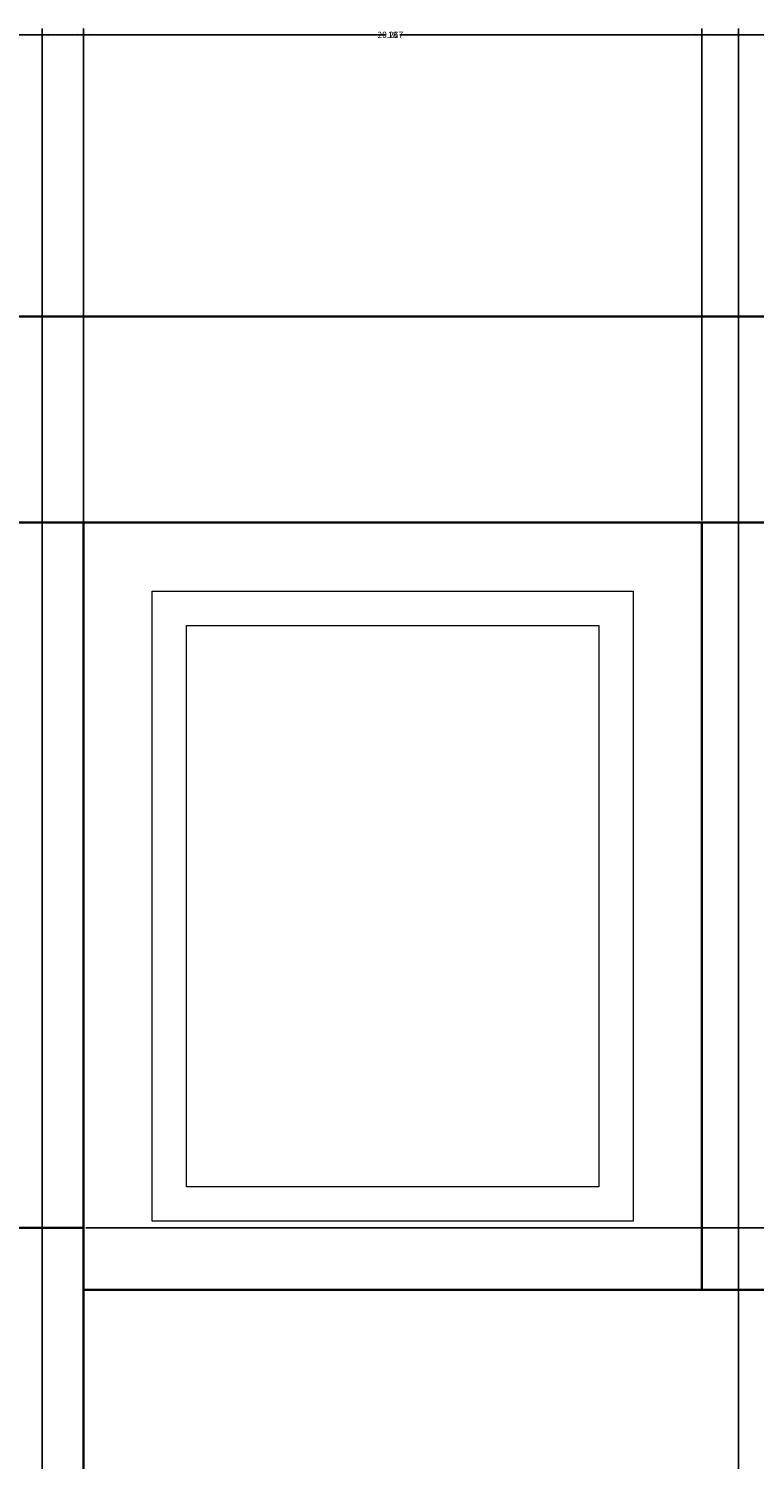
# Model space of a CAD drawing. Units: inches. Extents: x 27 to 200, y -50 to 102.
# Tile 24 of 26: x 145 to 166, y 61 to 102. Entities that reach past the tile are written whole.
import ezdxf

# ---------------------------------------------------------------- set-up
doc = ezdxf.new("R2010")
doc.units = ezdxf.units.IN
doc.header["$MEASUREMENT"] = 0
for name, color, linetype, lineweight in [('A-ANNO-DIMS', 2, 'Continuous', 18), ('A-ELEV', 7, 'Continuous', 35), ('A-FURN', 8, 'Continuous', 18)]:
    doc.layers.add(name, color=color, linetype=linetype, lineweight=lineweight)
doc.styles.get("Standard").update_dxf_attribs({"font": 'arial.ttf'})
doc.dimstyles.get("Standard").update_dxf_attribs({"dimtxt": 0.18, "dimasz": 0.18, "dimexe": 0.18, "dimexo": 0.0625, "dimgap": 0.09, "dimtad": 0, "dimtih": 1, "dimtoh": 1, "dimdec": 4, "dimzin": 0, "dimdsep": 46, "dimtxsty": 'Standard', "dimcen": 0.09, "dimadec": 0, "dimazin": 0, "dimtfac": 1, "dimtdec": 4, "dimtofl": 0, "dimtmove": 0, "dimatfit": 3, "dimfxl": 1, "dimtolj": 1, "dimtzin": 0, "dimarcsym": 0})

# ---------------------------------------------------------------- blocks, each defined once
blk = doc.blocks.new('CAB-DOOR-UPPER')
for p, q in [((0, 0), (0, 18.339)), ((0, 18.339), (14, 18.339)), ((14, 18.339), (14, 0)), ((1, 1), (1, 17.339)), ((1, 17.339), (13, 17.339)), ((13, 17.339), (13, 1)), ((13, 1), (1, 1)), ((14, 0), (0, 0))]:
    blk.add_line(p, q)
blk = doc.blocks.new('*D19')
at = {"layer": 'A-ANNO-DIMS', "color": 0, "lineweight": -2, "transparency": 16777216}
for p, q in [((133.417, 87.989), (133.417, 102.306)), ((133.597, 102.126), (139.706, 102.126)), ((146.237, 102.126), (140.127, 102.126)), ((146.417, 87.989), (146.417, 102.306))]:
    blk.add_line(p, q, dxfattribs=at)
at = {"layer": 'A-ANNO-DIMS', "color": 0, "transparency": 16777216}
for points in [[(133.597, 102.156), (133.597, 102.096), (133.417, 102.126)], [(146.237, 102.156), (146.237, 102.096), (146.417, 102.126)]]:
    blk.add_solid(points, dxfattribs=at)
at = {"layer": 'Defpoints', "color": 0, "transparency": 16777216}
for p in [(146.417, 102.126), (133.417, 87.926), (146.417, 87.926)]:
    blk.add_point(p, dxfattribs=at)
at = {"layer": 'A-ANNO-DIMS', "color": 0, "transparency": 16777216, "insert": (139.917, 102.126), "char_height": 0.18, "attachment_point": 5}
blk.add_mtext('\\A1;13', dxfattribs=at)
blk = doc.blocks.new('*D20')
at = {"layer": 'A-ANNO-DIMS', "color": 0, "lineweight": -2, "transparency": 16777216}
for p, q in [((146.417, 87.989), (146.417, 102.306)), ((146.597, 102.126), (155.206, 102.126)), ((164.237, 102.126), (155.628, 102.126)), ((164.417, 87.989), (164.417, 102.306))]:
    blk.add_line(p, q, dxfattribs=at)
at = {"layer": 'A-ANNO-DIMS', "color": 0, "transparency": 16777216}
for points in [[(146.597, 102.156), (146.597, 102.096), (146.417, 102.126)], [(164.237, 102.156), (164.237, 102.096), (164.417, 102.126)]]:
    blk.add_solid(points, dxfattribs=at)
at = {"layer": 'Defpoints', "color": 0, "transparency": 16777216}
for p in [(164.417, 102.126), (146.417, 87.926), (164.417, 87.926)]:
    blk.add_point(p, dxfattribs=at)
at = {"layer": 'A-ANNO-DIMS', "color": 0, "transparency": 16777216, "insert": (155.417, 102.126), "char_height": 0.18, "attachment_point": 5}
blk.add_mtext('\\A1;18', dxfattribs=at)
blk = doc.blocks.new('*D21')
at = {"layer": 'A-ANNO-DIMS', "color": 0, "lineweight": -2, "transparency": 16777216}
for p, q in [((164.417, 87.989), (164.417, 102.306)), ((164.597, 102.126), (173.206, 102.126)), ((182.237, 102.126), (173.628, 102.126)), ((182.417, 87.989), (182.417, 102.306))]:
    blk.add_line(p, q, dxfattribs=at)
at = {"layer": 'A-ANNO-DIMS', "color": 0, "transparency": 16777216}
for points in [[(164.597, 102.156), (164.597, 102.096), (164.417, 102.126)], [(182.237, 102.156), (182.237, 102.096), (182.417, 102.126)]]:
    blk.add_solid(points, dxfattribs=at)
at = {"layer": 'Defpoints', "color": 0, "transparency": 16777216}
for p in [(182.417, 102.126), (164.417, 87.926), (182.417, 87.926)]:
    blk.add_point(p, dxfattribs=at)
at = {"layer": 'A-ANNO-DIMS', "color": 0, "transparency": 16777216, "insert": (173.417, 102.126), "char_height": 0.18, "attachment_point": 5}
blk.add_mtext('\\A1;18', dxfattribs=at)
blk = doc.blocks.new('*D29')
at = {"layer": 'A-ANNO-DIMS', "color": 0, "lineweight": -2, "transparency": 16777216}
for p, q in [((146.479, 65.587), (199.797, 65.587)), ((199.617, 65.407), (199.617, 58.938)), ((199.617, 52.106), (199.617, 58.575)), ((146.479, 51.926), (199.797, 51.926))]:
    blk.add_line(p, q, dxfattribs=at)
at = {"layer": 'A-ANNO-DIMS', "color": 0, "transparency": 16777216}
for points in [[(199.587, 65.407), (199.647, 65.407), (199.617, 65.587)], [(199.587, 52.106), (199.647, 52.106), (199.617, 51.926)]]:
    blk.add_solid(points, dxfattribs=at)
at = {"layer": 'Defpoints', "color": 0, "transparency": 16777216}
for p in [(146.417, 65.587), (199.617, 65.587), (146.417, 51.926)]:
    blk.add_point(p, dxfattribs=at)
at = {"layer": 'A-ANNO-DIMS', "color": 0, "transparency": 16777216, "insert": (199.617, 58.756), "char_height": 0.18, "attachment_point": 5}
blk.add_mtext('\\A1;13.66', dxfattribs=at)
blk = doc.blocks.new('*D30')
at = {"layer": 'A-ANNO-DIMS', "color": 0, "lineweight": -2, "transparency": 16777216}
for p, q in [((146.479, 67.399), (199.797, 67.399)), ((199.617, 67.219), (199.617, 66.675)), ((199.617, 65.767), (199.617, 66.311)), ((146.479, 65.587), (199.797, 65.587))]:
    blk.add_line(p, q, dxfattribs=at)
at = {"layer": 'A-ANNO-DIMS', "color": 0, "transparency": 16777216}
for points in [[(199.587, 67.219), (199.647, 67.219), (199.617, 67.399)], [(199.587, 65.767), (199.647, 65.767), (199.617, 65.587)]]:
    blk.add_solid(points, dxfattribs=at)
at = {"layer": 'Defpoints', "color": 0, "transparency": 16777216}
for p in [(146.417, 67.399), (199.617, 67.399), (146.417, 65.587)]:
    blk.add_point(p, dxfattribs=at)
at = {"layer": 'A-ANNO-DIMS', "color": 0, "transparency": 16777216, "insert": (199.617, 66.493), "char_height": 0.18, "attachment_point": 5}
blk.add_mtext('\\A1;1.81', dxfattribs=at)
blk = doc.blocks.new('*D31')
at = {"layer": 'A-ANNO-DIMS', "color": 0, "lineweight": -2, "transparency": 16777216}
for p, q in [((146.479, 87.926), (199.797, 87.926)), ((199.617, 87.746), (199.617, 77.845)), ((199.617, 67.579), (199.617, 77.481)), ((146.479, 67.399), (199.797, 67.399))]:
    blk.add_line(p, q, dxfattribs=at)
at = {"layer": 'A-ANNO-DIMS', "color": 0, "transparency": 16777216}
for points in [[(199.587, 87.746), (199.647, 87.746), (199.617, 87.926)], [(199.587, 67.579), (199.647, 67.579), (199.617, 67.399)]]:
    blk.add_solid(points, dxfattribs=at)
at = {"layer": 'Defpoints', "color": 0, "transparency": 16777216}
for p in [(146.417, 87.926), (199.617, 87.926), (146.417, 67.399)]:
    blk.add_point(p, dxfattribs=at)
at = {"layer": 'A-ANNO-DIMS', "color": 0, "transparency": 16777216, "insert": (199.617, 77.663), "char_height": 0.18, "attachment_point": 5}
blk.add_mtext('\\A1;20.527', dxfattribs=at)
blk = doc.blocks.new('*D50')
at = {"layer": 'A-ANNO-DIMS', "color": 0, "lineweight": -2, "transparency": 16777216}
for p, q in [((138.722, 51.989), (138.722, 102.306)), ((138.902, 102.126), (142.176, 102.126)), ((146.237, 102.126), (142.963, 102.126)), ((146.417, 51.989), (146.417, 102.306))]:
    blk.add_line(p, q, dxfattribs=at)
at = {"layer": 'A-ANNO-DIMS', "color": 0, "transparency": 16777216}
for points in [[(138.902, 102.156), (138.902, 102.096), (138.722, 102.126)], [(146.237, 102.156), (146.237, 102.096), (146.417, 102.126)]]:
    blk.add_solid(points, dxfattribs=at)
at = {"layer": 'Defpoints', "color": 0, "transparency": 16777216}
for p in [(146.417, 102.126), (138.722, 51.926), (146.417, 51.926)]:
    blk.add_point(p, dxfattribs=at)
at = {"layer": 'A-ANNO-DIMS', "color": 0, "transparency": 16777216, "insert": (142.569, 102.126), "char_height": 0.18, "attachment_point": 5}
blk.add_mtext('\\A1;7.695', dxfattribs=at)
blk = doc.blocks.new('*D64')
at = {"layer": 'A-ANNO-DIMS', "color": 0, "lineweight": -2, "transparency": 16777216}
for p, q in [((145.216, 13.517), (145.216, 102.306)), ((145.396, 102.126), (154.884, 102.126)), ((165.303, 102.126), (155.815, 102.126)), ((165.483, 13.517), (165.483, 102.306))]:
    blk.add_line(p, q, dxfattribs=at)
at = {"layer": 'A-ANNO-DIMS', "color": 0, "transparency": 16777216}
for points in [[(145.396, 102.156), (145.396, 102.096), (145.216, 102.126)], [(165.303, 102.156), (165.303, 102.096), (165.483, 102.126)]]:
    blk.add_solid(points, dxfattribs=at)
at = {"layer": 'Defpoints', "color": 0, "transparency": 16777216}
for p in [(165.483, 102.126), (145.216, 13.455), (165.483, 13.455)]:
    blk.add_point(p, dxfattribs=at)
at = {"layer": 'A-ANNO-DIMS', "color": 0, "transparency": 16777216, "insert": (155.35, 102.126), "char_height": 0.18, "attachment_point": 5}
blk.add_mtext('\\A1;20.267', dxfattribs=at)

msp = doc.modelspace()

# ---------------------------------------------------------------- linework, layer by layer
at = {"layer": 'A-ELEV'}
for p, q in [((191.4169, 93.9264), (35.4169, 93.9264)), ((191.4169, 87.9264), (35.4169, 87.9264)), ((146.4169, 87.9264), (146.4169, 51.9264)), ((164.4169, 87.9264), (164.4169, 65.5865)), ((120.4169, 67.3991), (146.4169, 67.3991)), ((182.4169, 65.5865), (146.4169, 65.5865)), ((146.4169, 65.5865), (182.4169, 65.5865)), ((146.4169, 39.8559), (146.4169, 65.5865)), ((164.4169, 65.5865), (182.4169, 65.5865))]:
    msp.add_line(p, q, dxfattribs=at)

# ---------------------------------------------------------------- block references
at = {"layer": 'A-FURN'}
msp.add_blockref('CAB-DOOR-UPPER', (148.417, 67.587), dxfattribs=at)

# ---------------------------------------------------------------- dimensions: what is measured, and where the dimension line sits
at = {"layer": 'A-ANNO-DIMS'}
for base, p1, p2, override, picture, middle in [((146.4169, 102.1264), (133.4169, 87.9264), (146.4169, 87.9264), {"dimdec": 0, "dimlfac": 1, "dimrnd": 0, "dimzin": 0, "dimdsep": 46, "dimlunit": 2}, '*D19', (139.9169, 102.1264)), ((146.4169, 102.1264), (138.7218, 51.9264), (146.4169, 51.9264), {"dimdec": 3, "dimlfac": 1, "dimrnd": 0, "dimzin": 0, "dimdsep": 46, "dimlunit": 2}, '*D50', (142.5694, 102.1264)), ((165.4832, 102.1264), (145.216, 13.4548), (165.4832, 13.4548), {"dimdec": 3, "dimlfac": 1, "dimrnd": 0, "dimzin": 0, "dimdsep": 46, "dimlunit": 2}, '*D64', (155.3496, 102.1264)), ((164.4169, 102.1264), (146.4169, 87.9264), (164.4169, 87.9264), {"dimdec": 0, "dimlfac": 1, "dimrnd": 0, "dimzin": 0, "dimdsep": 46, "dimlunit": 2}, '*D20', (155.4169, 102.1264)), ((182.4169, 102.1264), (164.4169, 87.9264), (182.4169, 87.9264), {"dimdec": 0, "dimlfac": 1, "dimrnd": 0, "dimzin": 0, "dimdsep": 46, "dimlunit": 2}, '*D21', (173.4169, 102.1264))]:
    dim = msp.add_linear_dim(base=base, p1=p1, p2=p2, dimstyle='Standard', override=override, dxfattribs=at)
    dim.commit()
    dim.dimension.update_dxf_attribs({"geometry": picture, "text_midpoint": middle})
for base, p1, p2, override, picture, middle in [((199.6169, 87.9264), (146.4169, 67.3991), (146.4169, 87.9264), {"dimdec": 3, "dimlfac": 1, "dimrnd": 0, "dimzin": 0, "dimdsep": 46, "dimlunit": 2}, '*D31', (199.6169, 77.6628)), ((199.6169, 67.3991), (146.4169, 65.5865), (146.4169, 67.3991), {"dimdec": 2, "dimlfac": 1, "dimrnd": 0, "dimzin": 0, "dimdsep": 46, "dimlunit": 2}, '*D30', (199.6169, 66.4928)), ((199.6169, 65.5865), (146.4169, 51.9264), (146.4169, 65.5865), {"dimdec": 2, "dimlfac": 1, "dimrnd": 0, "dimzin": 0, "dimdsep": 46, "dimlunit": 2}, '*D29', (199.6169, 58.7565))]:
    dim = msp.add_linear_dim(base=base, p1=p1, p2=p2, angle=90, dimstyle='Standard', override=override, dxfattribs=at)
    dim.commit()
    dim.dimension.update_dxf_attribs({"geometry": picture, "text_midpoint": middle})

doc.saveas('drawing.dxf')
